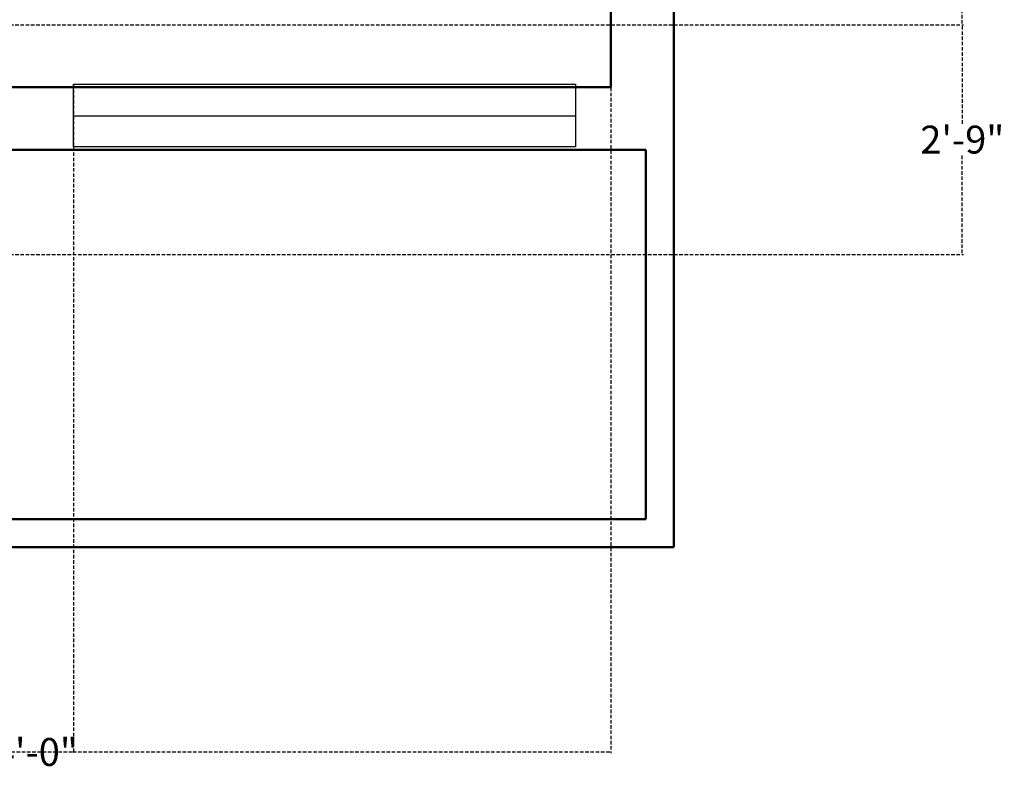
# Model space of a CAD drawing. Units: inches. Extents: x 513 to 1142, y 396 to 927.
# Tile 12 of 31: x 996 to 1137, y 399 to 507. Entities that reach past the tile are written whole.
import ezdxf

# ---------------------------------------------------------------- set-up
doc = ezdxf.new("R2010")
doc.units = ezdxf.units.IN
doc.header["$MEASUREMENT"] = 0
doc.linetypes.add('DASHED', pattern=[0.75, 0.5, -0.25])
for name, color, linetype, lineweight in [('A-ANNO-DIMS', 2, 'DASHED', 18), ('A-WALL', 7, 'Continuous', 50), ('windows', 172, 'Continuous', 25)]:
    doc.layers.add(name, color=color, linetype=linetype, lineweight=lineweight)
doc.styles.get("Standard").update_dxf_attribs({"font": 'arial.ttf'})
doc.dimstyles.get("Standard").update_dxf_attribs({"dimtxt": 4, "dimasz": 0.18, "dimexe": 0.18, "dimexo": 0.0625, "dimgap": 0.09, "dimtad": 0, "dimtih": 1, "dimtoh": 1, "dimdec": 0, "dimrnd": 6, "dimzin": 0, "dimdsep": 46, "dimlunit": 3, "dimtxsty": 'Standard', "dimcen": 0.09, "dimadec": 0, "dimazin": 0, "dimtfac": 1, "dimtdec": 0, "dimtofl": 0, "dimtmove": 0, "dimatfit": 3, "dimfxl": 1, "dimtolj": 1, "dimtzin": 0, "dimarcsym": 0})

# ---------------------------------------------------------------- blocks, each defined once
blk = doc.blocks.new('WIN-72IN')
blk.add_line((0, 4.45), (72, 4.45))
blk.add_lwpolyline([(72, 9), (72, 0), (0, 0), (0, 9)], close=True)
blk = doc.blocks.new('*D146')
at = {"layer": 'A-ANNO-DIMS', "color": 0, "lineweight": -2, "transparency": 16777216}
for p, q in [((913, 497.1), (913, 401.58)), ((1081, 497.1), (1081, 401.58)), ((913.18, 401.76), (990.22, 401.76)), ((1080.82, 401.76), (1003.77, 401.76))]:
    blk.add_line(p, q, dxfattribs=at)
at = {"layer": 'A-ANNO-DIMS', "color": 0, "transparency": 16777216}
for points in [[(913.18, 401.79), (913.18, 401.73), (913, 401.76)], [(1080.82, 401.79), (1080.82, 401.73), (1081, 401.76)]]:
    blk.add_solid(points, dxfattribs=at)
at = {"layer": 'Defpoints', "color": 0, "transparency": 16777216}
for p in [(913, 497.16), (1081, 497.16), (1081, 401.76)]:
    blk.add_point(p, dxfattribs=at)
at = {"layer": 'A-ANNO-DIMS', "color": 0, "transparency": 16777216, "insert": (997, 401.76), "char_height": 4, "attachment_point": 5}
blk.add_mtext('\\A1;14\'-0"', dxfattribs=at)
blk = doc.blocks.new('*D150')
at = {"layer": 'A-ANNO-DIMS', "color": 0, "lineweight": -2, "transparency": 16777216}
for p, q in [((904.06, 596.09), (1131.58, 596.09)), ((1131.4, 595.91), (1131.4, 553.23)), ((1131.4, 506.27), (1131.4, 548.96)), ((904.06, 506.09), (1131.58, 506.09))]:
    blk.add_line(p, q, dxfattribs=at)
at = {"layer": 'A-ANNO-DIMS', "color": 0, "transparency": 16777216}
for points in [[(1131.37, 595.91), (1131.43, 595.91), (1131.4, 596.09)], [(1131.37, 506.27), (1131.43, 506.27), (1131.4, 506.09)]]:
    blk.add_solid(points, dxfattribs=at)
at = {"layer": 'Defpoints', "color": 0, "transparency": 16777216}
for p in [(904, 596.09), (904, 506.09), (1131.4, 506.09)]:
    blk.add_point(p, dxfattribs=at)
at = {"layer": 'A-ANNO-DIMS', "color": 0, "transparency": 16777216, "insert": (1131.4, 551.09), "char_height": 4, "attachment_point": 5}
blk.add_mtext('\\A1;7\'-6"', dxfattribs=at)
blk = doc.blocks.new('*D158')
at = {"layer": 'A-ANNO-DIMS', "color": 0, "lineweight": -2, "transparency": 16777216}
for p, q in [((1003.92, 497.53), (1003.92, 401.58)), ((913, 497.1), (913, 401.58)), ((913.18, 401.76), (953.07, 401.76)), ((1003.74, 401.76), (963.85, 401.76))]:
    blk.add_line(p, q, dxfattribs=at)
at = {"layer": 'A-ANNO-DIMS', "color": 0, "transparency": 16777216}
for points in [[(913.18, 401.79), (913.18, 401.73), (913, 401.76)], [(1003.74, 401.79), (1003.74, 401.73), (1003.92, 401.76)]]:
    blk.add_solid(points, dxfattribs=at)
at = {"layer": 'Defpoints', "color": 0, "transparency": 16777216}
for p in [(913, 497.16), (1003.92, 497.6), (1003.92, 401.76)]:
    blk.add_point(p, dxfattribs=at)
at = {"layer": 'A-ANNO-DIMS', "color": 0, "transparency": 16777216, "insert": (958.46, 401.76), "char_height": 4, "attachment_point": 5}
blk.add_mtext('\\A1;7\'-7"', dxfattribs=at)
blk = doc.blocks.new('*D172')
at = {"layer": 'A-ANNO-DIMS', "color": 0, "lineweight": -2, "transparency": 16777216}
for p, q in [((904.06, 506.09), (1131.58, 506.09)), ((1131.4, 505.91), (1131.4, 491.76)), ((1131.4, 473.34), (1131.4, 487.49)), ((904.06, 473.16), (1131.58, 473.16))]:
    blk.add_line(p, q, dxfattribs=at)
at = {"layer": 'A-ANNO-DIMS', "color": 0, "transparency": 16777216}
for points in [[(1131.37, 505.91), (1131.43, 505.91), (1131.4, 506.09)], [(1131.37, 473.34), (1131.43, 473.34), (1131.4, 473.16)]]:
    blk.add_solid(points, dxfattribs=at)
at = {"layer": 'Defpoints', "color": 0, "transparency": 16777216}
for p in [(904, 506.09), (904, 473.16), (1131.4, 473.16)]:
    blk.add_point(p, dxfattribs=at)
at = {"layer": 'A-ANNO-DIMS', "color": 0, "transparency": 16777216, "insert": (1131.4, 489.63), "char_height": 4, "attachment_point": 5}
blk.add_mtext('\\A1;2\'-9"', dxfattribs=at)

msp = doc.modelspace()

# ---------------------------------------------------------------- linework, layer by layer
at = {"layer": 'A-WALL'}
for p, q in [((1090, 431.16), (1090, 879.16)), ((1081, 497.16), (1081, 637.16)), ((952.09, 497.16), (1081, 497.16)), ((952.09, 488.16), (1086, 488.16)), ((1086, 435.16), (1086, 488.16)), ((913, 435.16), (1086, 435.16)), ((909, 431.16), (1090, 431.16))]:
    msp.add_line(p, q, dxfattribs=at)

# ---------------------------------------------------------------- block references
at = {"layer": 'windows'}
msp.add_blockref('WIN-72IN', (1003.92, 488.6), dxfattribs=at)

# ---------------------------------------------------------------- dimensions: what is measured, and where the dimension line sits
at = {"layer": 'A-ANNO-DIMS'}
for base, p1, p2, picture, middle in [((1131.4, 506.09), (904, 596.09), (904, 506.09), '*D150', (1131.4, 551.09)), ((1131.4, 473.16), (904, 506.09), (904, 473.16), '*D172', (1131.4, 489.63))]:
    dim = msp.add_linear_dim(base=base, p1=p1, p2=p2, angle=90, dimstyle='Standard', override={"dimdec": 1, "dimlfac": 1, "dimrnd": 0, "dimzin": 1, "dimdsep": 46, "dimlunit": 4, "dimfrac": 2}, dxfattribs=at)
    dim.commit()
    dim.dimension.update_dxf_attribs({"geometry": picture, "text_midpoint": middle})
for base, p2, picture, middle in [((1003.92, 401.76), (1003.92, 497.6), '*D158', (958.46, 401.76)), ((1081, 401.76), (1081, 497.16), '*D146', (997, 401.76))]:
    dim = msp.add_linear_dim(base=base, p1=(913, 497.16), p2=p2, dimstyle='Standard', override={"dimdec": 1, "dimlfac": 1, "dimrnd": 0, "dimzin": 1, "dimdsep": 46, "dimlunit": 4, "dimfrac": 2}, dxfattribs=at)
    dim.commit()
    dim.dimension.update_dxf_attribs({"geometry": picture, "text_midpoint": middle})

doc.saveas('drawing.dxf')
